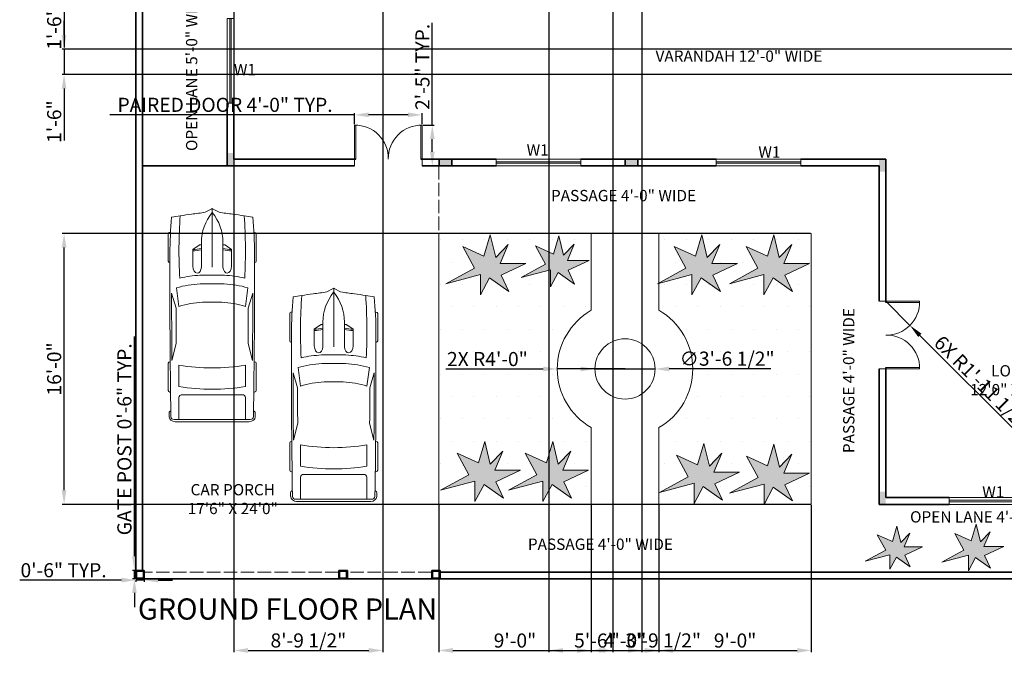
# Model space of a CAD drawing. Units: inches. Extents: x 13878 to 15021, y 3891 to 4810.
# Tile 1 of 3: x 13878 to 14576, y 3891 to 4347. Entities that reach past the tile are written whole.
import ezdxf

# ---------------------------------------------------------------- set-up
doc = ezdxf.new("R2010")
doc.units = ezdxf.units.IN
doc.linetypes.add('ACAD_ISO02W100', pattern=[15, 12, -3])
for name, color, linetype, lineweight in [('A-ANNO-DIMS', 2, 'Continuous', 18), ('A-ANNO-TEXT', 7, 'Continuous', 18), ('A-ANNO-TITL', 7, 'Continuous', 35), ('A-AREA-IDEN', 7, 'Continuous', 18), ('A-COLS', 7, 'Continuous', 35), ('A-COLS-PATT', 7, 'Continuous', 18), ('A-DOOR', 4, 'Continuous', 18), ('A-FLOR-OVHD', 220, 'ACAD_ISO02W100', 18), ('A-GLAZ', 4, 'Continuous', 18), ('A-WALL', 150, 'Continuous', 35), ('C-SITE-GATE', 220, 'ACAD_ISO02W100', 18), ('C-SITE-VEHI', 92, 'Continuous', 13), ('C-SITE-WALL', 150, 'Continuous', 35), ('L-PLNT', 85, 'Continuous', 18), ('L-PLNT-BEDS', 94, 'Continuous', 18)]:
    doc.layers.add(name, color=color, linetype=linetype, lineweight=lineweight)
doc.layers.add('L-PLNT-PATT', color=85, linetype='Continuous', lineweight=13, true_color=0x58ba48)
doc.styles.get("Standard").update_dxf_attribs({"font": 'arial.ttf'})
doc.dimstyles.new('ISO-25', dxfattribs={"dimtxt": 10, "dimasz": 10, "dimexe": 1.25, "dimexo": 0.625, "dimtad": 1, "dimdec": 0, "dimlunit": 3, "dimtxsty": 'Standard', "dimcen": 2.5, "dimadec": 0, "dimazin": 0, "dimtfac": 1, "dimtdec": 0, "dimtmove": 0, "dimatfit": 3, "dimfxl": 1, "dimarcsym": 0})

# ---------------------------------------------------------------- blocks, each defined once
blk = doc.blocks.new('*U2')
for p, q in [((536, 950), (536, 936)), ((1182, 988), (568, 988)), ((1214, 950), (1214, 950)), ((2235, 810), (1899, 912)), ((3412, 904), (3030, 807)), ((3440, 942), (3440, 950)), ((3472, 988), (4087, 988)), ((4119, 950), (4119, 934)), ((1779, 801), (2195, 746)), ((3516, 746), (3994, 746)), ((4179, 670), (4179, -670)), ((4736, 746), (4242, 746)), ((4736, -851), (4736, 851)), ((4785, -832), (4785, 832)), ((756, 241), (1313, 241)), ((816, 241), (816, 283)), ((820, 295), (918, 436)), ((918, 436), (1294, 436)), ((1496, -274), (1496, 274)), ((1690, -267), (1690, 267)), ((4736, -267), (4736, 267)), ((83, 156), (3, 10)), ((2102, 216), (2102, -216)), ((0, 0), (1313, 0)), ((3, -10), (83, -156)), ((756, -241), (1313, -241)), ((816, -241), (816, -283)), ((820, -295), (918, -436)), ((918, -436), (1294, -436)), ((2195, -746), (1779, -801)), ((2235, -810), (1899, -912)), ((3412, -904), (3030, -807)), ((3994, -746), (3516, -746)), ((4242, -746), (4736, -746)), ((536, -950), (536, -936)), ((1182, -988), (568, -988)), ((1214, -950), (1214, -950)), ((3440, -942), (3440, -950)), ((3472, -988), (4087, -988)), ((4119, -950), (4119, -934))]:
    blk.add_line(p, q)
for centre, major_axis, ratio, start_param, end_param in [((6757, -699), (0, 7958), 0.842304, 1.367076, 1.39176), ((1046, -12468), (0, 13417), 0.842304, 0.00281, 0.075598), ((568, 950), (0, -37.6), 0.842304, 3.141593, 4.712389), ((1638, -268113), (0, 269063), 0.842304, -0.013397, 0.002797), ((1182, 950), (0, 37.6), 0.842304, -1.570796, 0), ((1638, -268113), (0, -269025), 0.842304, 3.133765, 3.140441), ((3472, 950), (0, -37.6), 0.842304, 3.141593, 4.712389), ((4087, 950), (0, 37.6), 0.842304, -1.570796, 0), ((4588, 910), (0, 56.4), 0.842304, -0.013017, 1.249894), ((1638, -268131), (0, 269121), 0.842304, -0.013397, -0.013017), ((4673, 851), (0, -75.2), 0.842304, 1.570796, 3.128196), ((4673, 832), (0, -133), 0.842304, 1.570796, 3.128196), ((6583, -699), (0, -7755), 0.842304, 4.528606, 4.561838), ((952, -15087), (0, -15833), 0.842304, 3.096046, 3.200911), ((3414, 137), (0, -2280), 0.842304, 4.449482, 4.652344), ((3436, 137), (0, 2077), 0.842304, 1.245306, 1.50788), ((3800, 71), (0, -2021), 0.842304, 4.372215, 4.640744), ((2433, -93125), (0, -93935), 0.842304, 3.134049, 3.144098), ((434, 0), (0, 3734), 0.842304, 4.511394, 4.913384), ((912, 0), (0, 3734), 0.842304, 4.511394, 4.913384), ((4242, 670), (0, 75.2), 0.842304, 0, 1.570796), ((-5194, 1331), (0, -6374), 0.842304, 1.385369, 1.434372), ((756, -1185), (0, 1427), 0.842304, 0, 0.590319), ((832, 283), (0, 18.8), 0.842304, 0.879714, 1.570796), ((331, 432), (0, 696), 0.842304, 4.435146, 4.718221), ((361, 432), (0, 696), 0.842304, 4.435146, 4.718221), ((1290, 339), (161, -9), 0.603834, -1.395552, 1.581315), ((16, 0), (0, -18.8), 0.842304, 4.131459, 5.293319), ((-5194, -1331), (0, 6374), 0.842304, -1.434372, -1.385369), ((756, 1185), (0, 1427), 0.842304, 2.551274, 3.141593), ((3800, -71), (0, -2021), 0.842304, -1.499151, -1.230623), ((832, -283), (0, -18.8), 0.842304, 4.712389, 5.403472), ((331, -432), (0, -696), 0.842304, 1.564964, 1.848039), ((361, -432), (0, -696), 0.842304, 1.564964, 1.848039), ((3414, -137), (0, -2280), 0.842304, -1.510751, -1.307889), ((3436, -137), (0, -2077), 0.842304, -1.50788, -1.245306), ((6583, 699), (0, 7755), 0.842304, 1.721348, 1.754579), ((6757, 699), (0, 7958), 0.842304, 1.749832, 1.774517), ((952, 15087), (0, -15833), 0.842304, -0.059319, 0.045547), ((2433, 93125), (0, -93935), 0.842304, -0.002505, 0.007544), ((4242, -670), (0, -75.2), 0.842304, 4.712389, 6.283185), ((4673, -851), (0, 75.2), 0.842304, 3.15499, 4.712389), ((4673, -832), (0, -133), 0.842304, 0.013397, 1.570796), ((1046, 12468), (0, -13417), 0.842304, -0.075598, -0.00281), ((568, -950), (0, 37.6), 0.842304, 1.570796, 3.141593), ((1638, 268113), (0, 269063), 0.842304, 3.138796, 3.15499), ((1182, -950), (0, -37.6), 0.842304, 0, 1.570796), ((1638, 268113), (0, -269025), 0.842304, 0.001152, 0.007828), ((3472, -950), (0, -37.6), 0.842304, -1.570796, 0), ((4087, -950), (0, 37.6), 0.842304, 3.141593, 4.712389), ((4588, -910), (0, -56.4), 0.842304, -1.249894, 0.013017), ((1638, 268131), (0, 269121), 0.842304, 3.15461, 3.15499)]:
    blk.add_ellipse(centre, major_axis=major_axis, ratio=ratio, start_param=start_param, end_param=end_param)
at = {"extrusion": (0, 0, -1)}
blk.add_ellipse((1290, -339), major_axis=(161, 9), ratio=0.603834, start_param=-1.395552, end_param=1.581315, dxfattribs=at)
blk = doc.blocks.new('DOOR-PAIR-48IN')
for p, q in [((0, 48), (4.8, 48)), ((4.8, 48), (28.8, 48)), ((4.8, 47), (28.8, 47)), ((4.8, 1), (28.8, 1)), ((0, 0), (4.8, 0)), ((4.8, 0), (28.8, 0))]:
    blk.add_line(p, q)
for centre, start, end in [((5.3, 47.5), 268.78112, 1.21888), ((5.3, 0.5), 358.78112, 91.21888)]:
    blk.add_arc(centre, 23.51, start, end)
blk = doc.blocks.new('WINDOW-W1-60IN')
for p, q in [((0, 0), (0, 4.8)), ((0, 4.8), (60, 4.8)), ((0, 2.9), (60, 2.9)), ((0, 1.9), (60, 1.9)), ((60, 0), (60, 4.8)), ((0, 0), (60, 0))]:
    blk.add_line(p, q)
blk = doc.blocks.new('POST-GATE-6IN')
for p, q in [((6, 6), (0, 6)), ((0, 6), (0, 0)), ((5.5, 5.5), (0.5, 5.5)), ((0.5, 5.5), (0.5, 0.5)), ((0.5, 0.5), (5.5, 0.5)), ((5.5, 0.5), (5.5, 5.5)), ((6, 0), (6, 6)), ((0, 0), (6, 0))]:
    blk.add_line(p, q)
blk = doc.blocks.new('COLUMN-RECT-OUTLINED')
h = blk.add_hatch(color=256)
h.dxf.hatch_style = 1
h.paths.add_polyline_path([(9, 0), (9, 4.8), (0, 4.8), (0, 0)])
for p, q in [((0, 4.8), (0, 0)), ((9, 4.8), (0, 4.8)), ((9, 0), (9, 4.8)), ((0, 0), (9, 0))]:
    blk.add_line(p, q)
blk = doc.blocks.new('COLUMN-RECT-SOLID')
h = blk.add_hatch(color=256)
h.dxf.hatch_style = 1
h.paths.add_polyline_path([(0, 0), (4.8, 0), (4.8, 9), (0, 9)])
blk = doc.blocks.new('*D22')
at = {"layer": 'A-ANNO-DIMS', "color": 0, "lineweight": -2, "ltscale": 2, "transparency": 16777216}
for p, q in [((13959.74, 3966.66), (13959.74, 4122.53)), ((13960.01, 3956.66), (13958.49, 3956.66)), ((13959.74, 3950.66), (13959.74, 3956.66)), ((13960.01, 3950.66), (13958.49, 3950.66)), ((13959.74, 3940.66), (13959.74, 3930.66))]:
    blk.add_line(p, q, dxfattribs=at)
at = {"layer": 'A-ANNO-DIMS', "color": 0, "ltscale": 2, "transparency": 16777216}
for points in [[(13958.07, 3966.66), (13961.4, 3966.66), (13959.74, 3956.66)], [(13958.07, 3940.66), (13961.4, 3940.66), (13959.74, 3950.66)]]:
    blk.add_solid(points, dxfattribs=at)
at = {"layer": 'Defpoints', "color": 0, "ltscale": 2, "transparency": 16777216}
for p in [(13959.74, 3956.66), (13960.64, 3956.66), (13960.64, 3950.66)]:
    blk.add_point(p, dxfattribs=at)
at = {"layer": 'A-ANNO-DIMS', "color": 0, "ltscale": 2, "transparency": 16777216, "insert": (13953.94, 4049.6), "char_height": 10, "attachment_point": 5, "rotation": 90}
blk.add_mtext('GATE POST 0\'-6" TYP.', dxfattribs=at)
blk = doc.blocks.new('*D23')
at = {"layer": 'A-ANNO-DIMS', "color": 0, "lineweight": -2, "ltscale": 2, "transparency": 16777216}
for p, q in [((13950.64, 3949.76), (13878.43, 3949.76)), ((13960.64, 3950.03), (13960.64, 3948.51)), ((13966.64, 3949.76), (13960.64, 3949.76)), ((13966.64, 3950.03), (13966.64, 3948.51)), ((13976.64, 3949.76), (13986.64, 3949.76))]:
    blk.add_line(p, q, dxfattribs=at)
at = {"layer": 'A-ANNO-DIMS', "color": 0, "ltscale": 2, "transparency": 16777216}
for points in [[(13950.64, 3951.43), (13950.64, 3948.09), (13960.64, 3949.76)], [(13976.64, 3951.43), (13976.64, 3948.09), (13966.64, 3949.76)]]:
    blk.add_solid(points, dxfattribs=at)
at = {"layer": 'Defpoints', "color": 0, "ltscale": 2, "transparency": 16777216}
for p in [(13960.64, 3950.66), (13960.64, 3949.76), (13966.64, 3950.66)]:
    blk.add_point(p, dxfattribs=at)
at = {"layer": 'A-ANNO-DIMS', "color": 0, "ltscale": 2, "transparency": 16777216, "insert": (13909.54, 3955.49), "char_height": 10, "attachment_point": 5}
blk.add_mtext('0\'-6" TYP.', dxfattribs=at)
blk = doc.blocks.new('*D34')
at = {"layer": 'A-ANNO-DIMS', "color": 0, "lineweight": -2, "ltscale": 2, "transparency": 16777216}
for p, q in [((14115.67, 4279.6), (13942.28, 4279.6)), ((14115.67, 4273.02), (14115.67, 4280.85)), ((14153.67, 4279.6), (14125.67, 4279.6)), ((14163.67, 4273.02), (14163.67, 4280.85))]:
    blk.add_line(p, q, dxfattribs=at)
at = {"layer": 'A-ANNO-DIMS', "color": 0, "ltscale": 2, "transparency": 16777216}
for points in [[(14125.67, 4281.26), (14125.67, 4277.93), (14115.67, 4279.6)], [(14153.67, 4281.26), (14153.67, 4277.93), (14163.67, 4279.6)]]:
    blk.add_solid(points, dxfattribs=at)
at = {"layer": 'Defpoints', "color": 0, "ltscale": 2, "transparency": 16777216}
for p in [(14115.67, 4279.6), (14115.67, 4272.4), (14163.67, 4272.4)]:
    blk.add_point(p, dxfattribs=at)
at = {"layer": 'A-ANNO-DIMS', "color": 0, "ltscale": 2, "transparency": 16777216, "insert": (14023.98, 4285.4), "char_height": 10, "attachment_point": 5}
blk.add_mtext('PAIRED DOOR 4\'-0" TYP.', dxfattribs=at)
blk = doc.blocks.new('*D35')
at = {"layer": 'A-ANNO-DIMS', "color": 0, "lineweight": -2, "ltscale": 2, "transparency": 16777216}
for p, q in [((14170.87, 4272.4), (14170.87, 4344.77)), ((14164.3, 4272.4), (14172.12, 4272.4)), ((14170.87, 4253.46), (14170.87, 4262.4)), ((14164.3, 4243.46), (14172.12, 4243.46))]:
    blk.add_line(p, q, dxfattribs=at)
at = {"layer": 'A-ANNO-DIMS', "color": 0, "ltscale": 2, "transparency": 16777216}
for points in [[(14169.2, 4262.4), (14172.54, 4262.4), (14170.87, 4272.4)], [(14169.2, 4253.46), (14172.54, 4253.46), (14170.87, 4243.46)]]:
    blk.add_solid(points, dxfattribs=at)
at = {"layer": 'Defpoints', "color": 0, "ltscale": 2, "transparency": 16777216}
for p in [(14163.67, 4272.4), (14170.87, 4272.4), (14163.67, 4243.46)]:
    blk.add_point(p, dxfattribs=at)
at = {"layer": 'A-ANNO-DIMS', "color": 0, "ltscale": 2, "transparency": 16777216, "insert": (14165.14, 4313.58), "char_height": 10, "attachment_point": 5, "rotation": 90}
blk.add_mtext('2\'-5" TYP.', dxfattribs=at)
blk = doc.blocks.new('*D36')
at = {"layer": 'A-ANNO-DIMS', "color": 0, "lineweight": -2, "ltscale": 2, "transparency": 16777216}
for p, q in [((14030.24, 4466.43), (14030.24, 3898.66)), ((14135.84, 4466.43), (14135.84, 3898.66)), ((14040.24, 3899.91), (14125.84, 3899.91))]:
    blk.add_line(p, q, dxfattribs=at)
at = {"layer": 'A-ANNO-DIMS', "color": 0, "ltscale": 2, "transparency": 16777216}
for points in [[(14040.24, 3901.58), (14040.24, 3898.24), (14030.24, 3899.91)], [(14125.84, 3901.58), (14125.84, 3898.24), (14135.84, 3899.91)]]:
    blk.add_solid(points, dxfattribs=at)
at = {"layer": 'Defpoints', "color": 0, "ltscale": 2, "transparency": 16777216}
for p in [(14030.24, 4467.06), (14135.84, 4467.06), (14135.84, 3899.91)]:
    blk.add_point(p, dxfattribs=at)
at = {"layer": 'A-ANNO-DIMS', "color": 0, "ltscale": 2, "transparency": 16777216, "insert": (14083.04, 3905.71), "char_height": 10, "attachment_point": 5}
blk.add_mtext('8\'-9 1/2"', dxfattribs=at)
blk = doc.blocks.new('*D38')
at = {"layer": 'A-ANNO-DIMS', "color": 0, "lineweight": -2, "ltscale": 2, "transparency": 16777216}
for p, q in [((14253.44, 4612.43), (14253.44, 3898.66)), ((14319.44, 4612.43), (14319.44, 3898.66)), ((14263.44, 3899.91), (14309.44, 3899.91))]:
    blk.add_line(p, q, dxfattribs=at)
at = {"layer": 'A-ANNO-DIMS', "color": 0, "ltscale": 2, "transparency": 16777216}
for points in [[(14263.44, 3901.58), (14263.44, 3898.24), (14253.44, 3899.91)], [(14309.44, 3901.58), (14309.44, 3898.24), (14319.44, 3899.91)]]:
    blk.add_solid(points, dxfattribs=at)
at = {"layer": 'Defpoints', "color": 0, "ltscale": 2, "transparency": 16777216}
for p in [(14253.44, 4613.06), (14319.44, 4613.06), (14319.44, 3899.91)]:
    blk.add_point(p, dxfattribs=at)
at = {"layer": 'A-ANNO-DIMS', "color": 0, "ltscale": 2, "transparency": 16777216, "insert": (14286.44, 3905.64), "char_height": 10, "attachment_point": 5}
blk.add_mtext('5\'-6"', dxfattribs=at)
blk = doc.blocks.new('*D39')
at = {"layer": 'A-ANNO-DIMS', "color": 0, "lineweight": -2, "ltscale": 2, "transparency": 16777216}
for p, q in [((14253.44, 4396.43), (14253.44, 3898.66)), ((14298.9, 4396.43), (14298.9, 3898.66)), ((14263.44, 3899.91), (14288.9, 3899.91)), ((14298.9, 3899.91), (14360.03, 3899.91))]:
    blk.add_line(p, q, dxfattribs=at)
at = {"layer": 'A-ANNO-DIMS', "color": 0, "ltscale": 2, "transparency": 16777216}
for points in [[(14263.44, 3901.58), (14263.44, 3898.24), (14253.44, 3899.91)], [(14288.9, 3901.58), (14288.9, 3898.24), (14298.9, 3899.91)]]:
    blk.add_solid(points, dxfattribs=at)
at = {"layer": 'Defpoints', "color": 0, "ltscale": 2, "transparency": 16777216}
for p in [(14253.44, 4397.06), (14298.9, 4397.06), (14298.9, 3899.91)]:
    blk.add_point(p, dxfattribs=at)
at = {"layer": 'A-ANNO-DIMS', "color": 0, "ltscale": 2, "transparency": 16777216, "insert": (14334.46, 3905.71), "char_height": 10, "attachment_point": 5}
blk.add_mtext('3\'-9 1/2"', dxfattribs=at)
blk = doc.blocks.new('*D40')
at = {"layer": 'A-ANNO-DIMS', "color": 0, "lineweight": -2, "ltscale": 2, "transparency": 16777216}
for p, q in [((13909.89, 4402.26), (13909.89, 4412.26)), ((14838.41, 4392.26), (13908.64, 4392.26)), ((13909.89, 4392.26), (13909.89, 4374.26)), ((14838.41, 4374.26), (13908.64, 4374.26)), ((13909.89, 4364.26), (13909.89, 4327.37))]:
    blk.add_line(p, q, dxfattribs=at)
at = {"layer": 'A-ANNO-DIMS', "color": 0, "ltscale": 2, "transparency": 16777216}
for points in [[(13908.22, 4402.26), (13911.55, 4402.26), (13909.89, 4392.26)], [(13908.22, 4364.26), (13911.55, 4364.26), (13909.89, 4374.26)]]:
    blk.add_solid(points, dxfattribs=at)
at = {"layer": 'Defpoints', "color": 0, "ltscale": 2, "transparency": 16777216}
for p in [(14839.04, 4392.26), (13909.89, 4374.26), (14839.04, 4374.26)]:
    blk.add_point(p, dxfattribs=at)
at = {"layer": 'A-ANNO-DIMS', "color": 0, "ltscale": 2, "transparency": 16777216, "insert": (13904.16, 4340.81), "char_height": 10, "attachment_point": 5, "rotation": 90}
blk.add_mtext('1\'-6"', dxfattribs=at)
blk = doc.blocks.new('*D41')
at = {"layer": 'A-ANNO-DIMS', "color": 0, "lineweight": -2, "ltscale": 2, "transparency": 16777216}
for p, q in [((13909.89, 4336.26), (13909.89, 4346.26)), ((14838.41, 4326.26), (13908.64, 4326.26)), ((13909.89, 4326.26), (13909.89, 4308.26)), ((14838.41, 4308.26), (13908.64, 4308.26)), ((13909.89, 4298.26), (13909.89, 4261.37))]:
    blk.add_line(p, q, dxfattribs=at)
at = {"layer": 'A-ANNO-DIMS', "color": 0, "ltscale": 2, "transparency": 16777216}
for points in [[(13908.22, 4336.26), (13911.55, 4336.26), (13909.89, 4326.26)], [(13908.22, 4298.26), (13911.55, 4298.26), (13909.89, 4308.26)]]:
    blk.add_solid(points, dxfattribs=at)
at = {"layer": 'Defpoints', "color": 0, "ltscale": 2, "transparency": 16777216}
for p in [(14839.04, 4326.26), (13909.89, 4308.26), (14839.04, 4308.26)]:
    blk.add_point(p, dxfattribs=at)
at = {"layer": 'A-ANNO-DIMS', "color": 0, "ltscale": 2, "transparency": 16777216, "insert": (13904.16, 4274.81), "char_height": 10, "attachment_point": 5, "rotation": 90}
blk.add_mtext('1\'-6"', dxfattribs=at)
blk = doc.blocks.new('*D42')
at = {"layer": 'A-ANNO-DIMS', "color": 0, "lineweight": -2, "ltscale": 2, "transparency": 16777216}
for p, q in [((14175.44, 4002.83), (14175.44, 3898.66)), ((14283.44, 4002.83), (14283.44, 3898.66)), ((14185.44, 3899.91), (14273.44, 3899.91))]:
    blk.add_line(p, q, dxfattribs=at)
at = {"layer": 'A-ANNO-DIMS', "color": 0, "ltscale": 2, "transparency": 16777216}
for points in [[(14185.44, 3901.58), (14185.44, 3898.24), (14175.44, 3899.91)], [(14273.44, 3901.58), (14273.44, 3898.24), (14283.44, 3899.91)]]:
    blk.add_solid(points, dxfattribs=at)
at = {"layer": 'Defpoints', "color": 0, "ltscale": 2, "transparency": 16777216}
for p in [(14175.44, 4003.46), (14283.44, 4003.46), (14283.44, 3899.91)]:
    blk.add_point(p, dxfattribs=at)
at = {"layer": 'A-ANNO-DIMS', "color": 0, "ltscale": 2, "transparency": 16777216, "insert": (14229.44, 3905.64), "char_height": 10, "attachment_point": 5}
blk.add_mtext('9\'-0"', dxfattribs=at)
blk = doc.blocks.new('*D43')
at = {"layer": 'A-ANNO-DIMS', "color": 0, "lineweight": -2, "ltscale": 2, "transparency": 16777216}
for p, q in [((14283.44, 4002.83), (14283.44, 3898.66)), ((14331.44, 4002.83), (14331.44, 3898.66)), ((14293.44, 3899.91), (14321.44, 3899.91))]:
    blk.add_line(p, q, dxfattribs=at)
at = {"layer": 'A-ANNO-DIMS', "color": 0, "ltscale": 2, "transparency": 16777216}
for points in [[(14293.44, 3901.58), (14293.44, 3898.24), (14283.44, 3899.91)], [(14321.44, 3901.58), (14321.44, 3898.24), (14331.44, 3899.91)]]:
    blk.add_solid(points, dxfattribs=at)
at = {"layer": 'Defpoints', "color": 0, "ltscale": 2, "transparency": 16777216}
for p in [(14283.44, 4003.46), (14331.44, 4003.46), (14331.44, 3899.91)]:
    blk.add_point(p, dxfattribs=at)
at = {"layer": 'A-ANNO-DIMS', "color": 0, "ltscale": 2, "transparency": 16777216, "insert": (14307.44, 3905.64), "char_height": 10, "attachment_point": 5}
blk.add_mtext('4\'-0"', dxfattribs=at)
blk = doc.blocks.new('*D44')
at = {"layer": 'A-ANNO-DIMS', "color": 0, "lineweight": -2, "ltscale": 2, "transparency": 16777216}
for p, q in [((14331.44, 4002.83), (14331.44, 3898.66)), ((14439.44, 4002.83), (14439.44, 3898.66)), ((14341.44, 3899.91), (14429.44, 3899.91))]:
    blk.add_line(p, q, dxfattribs=at)
at = {"layer": 'A-ANNO-DIMS', "color": 0, "ltscale": 2, "transparency": 16777216}
for points in [[(14341.44, 3901.58), (14341.44, 3898.24), (14331.44, 3899.91)], [(14429.44, 3901.58), (14429.44, 3898.24), (14439.44, 3899.91)]]:
    blk.add_solid(points, dxfattribs=at)
at = {"layer": 'Defpoints', "color": 0, "ltscale": 2, "transparency": 16777216}
for p in [(14331.44, 4003.46), (14439.44, 4003.46), (14439.44, 3899.91)]:
    blk.add_point(p, dxfattribs=at)
at = {"layer": 'A-ANNO-DIMS', "color": 0, "ltscale": 2, "transparency": 16777216, "insert": (14385.44, 3905.64), "char_height": 10, "attachment_point": 5}
blk.add_mtext('9\'-0"', dxfattribs=at)
blk = doc.blocks.new('*D45')
at = {"layer": 'A-ANNO-DIMS', "color": 0, "lineweight": -2, "ltscale": 2, "transparency": 16777216}
for p, q in [((14438.81, 4195.46), (13908.64, 4195.46)), ((13909.89, 4013.46), (13909.89, 4185.46)), ((14438.81, 4003.46), (13908.64, 4003.46))]:
    blk.add_line(p, q, dxfattribs=at)
at = {"layer": 'A-ANNO-DIMS', "color": 0, "ltscale": 2, "transparency": 16777216}
for points in [[(13908.22, 4185.46), (13911.55, 4185.46), (13909.89, 4195.46)], [(13908.22, 4013.46), (13911.55, 4013.46), (13909.89, 4003.46)]]:
    blk.add_solid(points, dxfattribs=at)
at = {"layer": 'Defpoints', "color": 0, "ltscale": 2, "transparency": 16777216}
for p in [(13909.89, 4195.46), (14439.44, 4195.46), (14439.44, 4003.46)]:
    blk.add_point(p, dxfattribs=at)
at = {"layer": 'A-ANNO-DIMS', "color": 0, "ltscale": 2, "transparency": 16777216, "insert": (13904.16, 4099.46), "char_height": 10, "attachment_point": 5, "rotation": 90}
blk.add_mtext('16\'-0"', dxfattribs=at)
blk = doc.blocks.new('*D46')
at = {"layer": 'A-ANNO-DIMS', "color": 0, "lineweight": -2, "ltscale": 2, "transparency": 16777216}
for p, q in [((14180.38, 4099.46), (14249.44, 4099.46)), ((14307.44, 4099.46), (14259.44, 4099.46))]:
    blk.add_line(p, q, dxfattribs=at)
at = {"layer": 'A-ANNO-DIMS', "color": 0, "ltscale": 2, "transparency": 16777216}
blk.add_solid([(14249.44, 4101.13), (14249.44, 4097.79), (14259.44, 4099.46)], dxfattribs=at)
at = {"layer": 'Defpoints', "color": 0, "ltscale": 2, "transparency": 16777216}
for p in [(14259.44, 4099.46), (14307.44, 4099.46)]:
    blk.add_point(p, dxfattribs=at)
at = {"layer": 'A-ANNO-DIMS', "color": 0, "ltscale": 2, "transparency": 16777216, "insert": (14209.91, 4105.19), "char_height": 10, "attachment_point": 5, "rotation": 359.99979}
blk.add_mtext('2X R4\'-0"', dxfattribs=at)
blk = doc.blocks.new('*D47')
at = {"layer": 'A-ANNO-DIMS', "color": 0, "lineweight": -2, "ltscale": 2, "transparency": 16777216}
for p, q in [((14276.09, 4099.46), (14266.09, 4099.46)), ((14286.09, 4099.46), (14328.79, 4099.46)), ((14410.8, 4099.46), (14338.79, 4099.46))]:
    blk.add_line(p, q, dxfattribs=at)
at = {"layer": 'A-ANNO-DIMS', "color": 0, "ltscale": 2, "transparency": 16777216}
for points in [[(14276.09, 4101.13), (14276.09, 4097.79), (14286.09, 4099.46)], [(14338.79, 4101.13), (14338.79, 4097.79), (14328.79, 4099.46)]]:
    blk.add_solid(points, dxfattribs=at)
at = {"layer": 'Defpoints', "color": 0, "ltscale": 2, "transparency": 16777216}
for p in [(14286.09, 4099.46), (14328.79, 4099.46)]:
    blk.add_point(p, dxfattribs=at)
at = {"layer": 'A-ANNO-DIMS', "color": 0, "ltscale": 2, "transparency": 16777216, "insert": (14379.79, 4105.47), "char_height": 10, "attachment_point": 5, "rotation": 0.00046}
blk.add_mtext('∅3\'-6 1/2"', dxfattribs=at)
blk = doc.blocks.new('*D50')
at = {"layer": 'A-ANNO-DIMS', "color": 0, "lineweight": -2, "ltscale": 2, "transparency": 16777216}
for p, q in [((14492.74, 4146.96), (14509.36, 4130.34)), ((14587.15, 4052.55), (14516.43, 4123.27))]:
    blk.add_line(p, q, dxfattribs=at)
at = {"layer": 'A-ANNO-DIMS', "color": 0, "ltscale": 2, "transparency": 16777216}
blk.add_solid([(14517.61, 4124.45), (14515.25, 4122.09), (14509.36, 4130.34)], dxfattribs=at)
at = {"layer": 'Defpoints', "color": 0, "ltscale": 2, "transparency": 16777216}
for p in [(14492.74, 4146.96), (14509.36, 4130.34)]:
    blk.add_point(p, dxfattribs=at)
at = {"layer": 'A-ANNO-DIMS', "color": 0, "ltscale": 2, "transparency": 16777216, "insert": (14559.42, 4088.47), "char_height": 10, "attachment_point": 5, "rotation": 315.00023}
blk.add_mtext('6X R1\'-11 1/2"', dxfattribs=at)

msp = doc.modelspace()

# ---------------------------------------------------------------- hatches: boundary and pattern name
at = {"layer": 'L-PLNT-PATT'}
h = msp.add_hatch(dxfattribs=at)
h.set_pattern_fill('DOTS', color=256, scale=10)
h.paths.add_polyline_path([(14283.44, 4141.03), (14283.44, 4195.46), (14175.44, 4195.46), (14175.44, 4003.46), (14283.44, 4003.46), (14283.44, 4057.89, -0.57735)])
h.paths.add_polyline_path([(14225.1, 4154.41), (14211.42, 4164.09), (14204.93, 4151.94), (14204.93, 4166.36), (14180.44, 4159.88), (14200.72, 4170.9), (14192.4, 4186.2), (14207.36, 4179.33), (14211.91, 4194.56), (14215.8, 4178.36), (14224.72, 4187.59), (14219.04, 4174.14), (14237.21, 4174.14), (14219.69, 4165.88)], flags=16)
h.paths.add_polyline_path([(14233.76, 4164.32), (14251, 4173.69), (14243.93, 4186.7), (14256.65, 4180.86), (14260.52, 4193.82), (14263.83, 4180.03), (14271.41, 4187.89), (14266.58, 4176.45), (14282.03, 4176.45), (14267.14, 4169.42), (14271.74, 4159.67), (14260.1, 4167.9), (14254.58, 4157.57), (14254.58, 4169.83)], flags=16)
h.paths.add_polyline_path([(14208.03, 4048.13), (14211.93, 4031.92), (14220.85, 4041.16), (14215.17, 4027.71), (14233.33, 4027.71), (14215.82, 4019.44), (14221.23, 4007.98), (14207.55, 4017.66), (14201.06, 4005.5), (14201.06, 4019.93), (14176.57, 4013.45), (14196.84, 4024.47), (14188.53, 4039.77), (14203.49, 4032.89)], flags=16)
h.paths.add_polyline_path([(14256.22, 4048.13), (14260.11, 4031.92), (14269.03, 4041.16), (14263.36, 4027.71), (14281.52, 4027.71), (14264.01, 4019.44), (14269.42, 4007.98), (14255.74, 4017.66), (14249.25, 4005.5), (14249.25, 4019.93), (14224.76, 4013.45), (14245.03, 4024.47), (14236.72, 4039.77), (14251.68, 4032.89)], flags=16)
h = msp.add_hatch(color=256, dxfattribs=at)
h.dxf.hatch_style = 1
h.paths.add_polyline_path([(14211.42, 4164.09), (14225.1, 4154.41), (14219.69, 4165.88), (14237.21, 4174.14), (14219.04, 4174.14), (14224.72, 4187.59), (14215.8, 4178.36), (14211.91, 4194.56), (14207.36, 4179.33), (14192.4, 4186.2), (14200.72, 4170.9), (14180.44, 4159.88), (14204.93, 4166.36), (14204.93, 4151.94)])
h.paths.add_polyline_path([(14260.1, 4167.9), (14271.74, 4159.67), (14267.14, 4169.42), (14282.03, 4176.45), (14266.58, 4176.45), (14271.41, 4187.89), (14263.83, 4180.03), (14260.52, 4193.82), (14256.65, 4180.86), (14243.93, 4186.7), (14251, 4173.69), (14233.76, 4164.32), (14254.58, 4169.83), (14254.58, 4157.57)])
h.paths.add_polyline_path([(14365.73, 4178.36), (14361.84, 4194.56), (14357.3, 4179.33), (14342.33, 4186.2), (14350.65, 4170.9), (14331.44, 4160.46), (14331.44, 4160.16), (14354.86, 4166.36), (14354.86, 4151.94), (14361.35, 4164.09), (14375.03, 4154.41), (14369.62, 4165.88), (14387.14, 4174.14), (14368.97, 4174.14), (14374.65, 4187.59)])
h.paths.add_polyline_path([(14420, 4174.14), (14425.67, 4187.59), (14416.75, 4178.36), (14412.86, 4194.56), (14408.32, 4179.33), (14393.35, 4186.2), (14401.67, 4170.9), (14381.4, 4159.88), (14405.89, 4166.36), (14405.89, 4151.94), (14412.37, 4164.09), (14426.05, 4154.41), (14420.65, 4165.88), (14438.16, 4174.14)])
h.paths.add_polyline_path([(14249.25, 4019.93), (14249.25, 4005.5), (14255.74, 4017.66), (14269.42, 4007.98), (14264.01, 4019.44), (14281.52, 4027.71), (14263.36, 4027.71), (14269.03, 4041.16), (14260.11, 4031.92), (14256.22, 4048.13), (14251.68, 4032.89), (14236.72, 4039.77), (14245.03, 4024.47), (14224.76, 4013.45)])
h.paths.add_polyline_path([(14203.49, 4032.89), (14188.53, 4039.77), (14196.84, 4024.47), (14176.57, 4013.45), (14201.06, 4019.93), (14201.06, 4005.5), (14207.55, 4017.66), (14221.23, 4007.98), (14215.82, 4019.44), (14233.33, 4027.71), (14215.17, 4027.71), (14220.85, 4041.16), (14211.93, 4031.92), (14208.03, 4048.13)])
h.paths.add_polyline_path([(14362.82, 4016.2), (14376.5, 4006.52), (14371.09, 4017.98), (14388.61, 4026.25), (14370.44, 4026.25), (14376.12, 4039.7), (14367.2, 4030.46), (14363.31, 4046.67), (14358.76, 4031.44), (14343.8, 4038.31), (14352.12, 4023.01), (14331.84, 4011.99), (14356.33, 4018.47), (14356.33, 4004.05)])
h.paths.add_polyline_path([(14408.41, 4030.85), (14393.45, 4037.72), (14401.76, 4022.42), (14381.49, 4011.4), (14405.98, 4017.88), (14405.98, 4003.46), (14412.47, 4015.62), (14426.15, 4005.94), (14420.74, 4017.4), (14438.25, 4025.66), (14420.09, 4025.66), (14425.77, 4039.12), (14416.85, 4029.88), (14412.95, 4046.08)])
h.paths.add_polyline_path([(14502.95, 3976.33), (14500.16, 3987.92), (14496.92, 3977.03), (14486.21, 3981.94), (14492.16, 3971), (14477.66, 3963.12), (14495.18, 3967.76), (14495.18, 3957.44), (14499.81, 3966.13), (14509.6, 3959.21), (14505.73, 3967.41), (14518.25, 3973.32), (14505.27, 3973.32), (14509.32, 3982.94)])
h.paths.add_polyline_path([(14552.74, 3977.57), (14541.18, 3982.88), (14547.61, 3971.06), (14531.95, 3962.55), (14550.86, 3967.56), (14550.86, 3956.41), (14555.87, 3965.8), (14566.44, 3958.33), (14562.26, 3967.18), (14575.79, 3973.56), (14561.76, 3973.56), (14566.15, 3983.95), (14559.26, 3976.82), (14556.25, 3989.34)])
h.paths.add_polyline_path([(14605.39, 3973.1), (14587.22, 3963.23), (14609.17, 3969.04), (14609.17, 3956.11), (14614.98, 3967), (14627.25, 3958.33), (14622.4, 3968.6), (14638.1, 3976.01), (14621.82, 3976.01), (14626.9, 3988.07), (14618.91, 3979.79), (14615.42, 3994.31), (14611.35, 3980.66), (14597.94, 3986.82)])
h = msp.add_hatch(dxfattribs=at)
h.set_pattern_fill('DOTS', color=256, scale=10)
h.paths.add_polyline_path([(14439.44, 4195.46), (14331.44, 4195.46), (14331.44, 4160.46), (14350.65, 4170.9), (14342.33, 4186.2), (14357.3, 4179.33), (14361.84, 4194.56), (14365.73, 4178.36), (14374.65, 4187.59), (14368.97, 4174.14), (14387.14, 4174.14), (14369.62, 4165.88), (14375.03, 4154.41), (14361.35, 4164.09), (14354.86, 4151.94), (14354.86, 4166.36), (14331.44, 4160.16), (14331.44, 4141.03, -0.57735), (14331.44, 4057.89), (14331.44, 4003.46), (14405.98, 4003.46), (14405.98, 4017.88), (14381.49, 4011.4), (14401.76, 4022.42), (14393.45, 4037.72), (14408.41, 4030.85), (14412.95, 4046.08), (14416.85, 4029.88), (14425.77, 4039.12), (14420.09, 4025.66), (14438.25, 4025.66), (14420.74, 4017.4), (14426.15, 4005.94), (14412.47, 4015.62), (14405.98, 4003.46), (14439.44, 4003.46)])
h.paths.add_polyline_path([(14381.4, 4159.88), (14401.67, 4170.9), (14393.35, 4186.2), (14408.32, 4179.33), (14412.86, 4194.56), (14416.75, 4178.36), (14425.67, 4187.59), (14420, 4174.14), (14438.16, 4174.14), (14420.65, 4165.88), (14426.05, 4154.41), (14412.37, 4164.09), (14405.89, 4151.94), (14405.89, 4166.36)], flags=16)
h.paths.add_polyline_path([(14363.31, 4046.67), (14367.2, 4030.46), (14376.12, 4039.7), (14370.44, 4026.25), (14388.61, 4026.25), (14371.09, 4017.98), (14376.5, 4006.52), (14362.82, 4016.2), (14356.33, 4004.05), (14356.33, 4018.47), (14331.84, 4011.99), (14352.12, 4023.01), (14343.8, 4038.31), (14358.76, 4031.44)], flags=16)

# ---------------------------------------------------------------- linework, layer by layer
at = {"layer": 'A-DOOR'}
for p, q in [((14487.44, 4147.46), (14492.24, 4147.46)), ((14492.24, 4147.46), (14516.24, 4147.46)), ((14492.24, 4146.46), (14516.24, 4146.46)), ((14492.24, 4123.45), (14492.24, 4123.46)), ((14487.44, 4099.46), (14492.24, 4099.46)), ((14492.24, 4100.46), (14516.24, 4100.46)), ((14492.24, 4099.46), (14516.24, 4099.46))]:
    msp.add_line(p, q, dxfattribs=at)
for centre, radius, start, end in [((14492.74, 4146.96), 23.51, 268.78112, 1.21888), ((14492.74, 4099.96), 23.5, 358.78085, 91.23184)]:
    msp.add_arc(centre, radius, start, end, dxfattribs=at)
at = {"layer": 'A-FLOR-OVHD', "ltscale": 0.8}
msp.add_line((14175.44, 4243.46), (14175.44, 3956.66), dxfattribs=at)
at = {"layer": 'A-GLAZ'}
msp.add_line((14216.1, 4246.36), (14276.1, 4246.36), dxfattribs=at)
at = {"layer": 'A-WALL'}
for p, q in [((14025.44, 4243.46), (14025.44, 4287.86)), ((14030.24, 4248.26), (14030.24, 4287.86)), ((14115.67, 4243.46), (13965.44, 4243.46)), ((14116.67, 4248.26), (14030.24, 4248.26)), ((14216.1, 4248.26), (14162.67, 4248.26)), ((14184.77, 4243.46), (14163.67, 4243.46)), ((14216.1, 4243.46), (14184.77, 4243.46)), ((14371.94, 4248.26), (14276.1, 4248.26)), ((14307.44, 4243.46), (14276.1, 4243.46)), ((14316.44, 4243.46), (14307.44, 4243.46)), ((14371.94, 4243.46), (14316.44, 4243.46)), ((14492.24, 4248.26), (14431.94, 4248.26)), ((14487.44, 4243.46), (14431.94, 4243.46)), ((14487.44, 4147.46), (14487.44, 4243.46)), ((14492.24, 4146.46), (14492.24, 4248.26)), ((14487.44, 4003.46), (14487.44, 4099.46)), ((14492.24, 4008.26), (14492.24, 4100.46)), ((14537.24, 4008.26), (14492.24, 4008.26)), ((14537.24, 4003.46), (14487.44, 4003.46))]:
    msp.add_line(p, q, dxfattribs=at)
at = {"layer": 'C-SITE-GATE', "ltscale": 0.8}
for p, q in [((14104.64, 3955.46), (13966.64, 3955.46)), ((14170.41, 3955.46), (14110.64, 3955.46))]:
    msp.add_line(p, q, dxfattribs=at)
at = {"layer": 'C-SITE-WALL'}
for p, q in [((13960.64, 3950.66), (13960.64, 4670.66)), ((13965.44, 3956.66), (13965.44, 4392.26)), ((13966.64, 3950.66), (13960.64, 3950.66)), ((14176.41, 3950.66), (13966.64, 3950.66)), ((14487.44, 3955.46), (14176.41, 3955.46)), ((14920.64, 3950.66), (14176.41, 3950.66)), ((14642.24, 3955.46), (14487.44, 3955.46))]:
    msp.add_line(p, q, dxfattribs=at)
at = {"layer": 'L-PLNT'}
for p, q in [((14207.36, 4179.33), (14211.91, 4194.56)), ((14211.91, 4194.56), (14215.8, 4178.36)), ((14256.65, 4180.86), (14260.52, 4193.82)), ((14260.52, 4193.82), (14263.83, 4180.03)), ((14357.3, 4179.33), (14361.84, 4194.56)), ((14361.84, 4194.56), (14365.73, 4178.36)), ((14408.32, 4179.33), (14412.86, 4194.56)), ((14412.86, 4194.56), (14416.75, 4178.36)), ((14215.8, 4178.36), (14224.72, 4187.59)), ((14224.72, 4187.59), (14219.04, 4174.14)), ((14263.83, 4180.03), (14271.41, 4187.89)), ((14271.41, 4187.89), (14266.58, 4176.45)), ((14365.73, 4178.36), (14374.65, 4187.59)), ((14374.65, 4187.59), (14368.97, 4174.14)), ((14416.75, 4178.36), (14425.67, 4187.59)), ((14425.67, 4187.59), (14420, 4174.14)), ((14200.72, 4170.9), (14192.4, 4186.2)), ((14192.4, 4186.2), (14207.36, 4179.33)), ((14251, 4173.69), (14243.93, 4186.7)), ((14243.93, 4186.7), (14256.65, 4180.86)), ((14350.65, 4170.9), (14342.33, 4186.2)), ((14342.33, 4186.2), (14357.3, 4179.33)), ((14401.67, 4170.9), (14393.35, 4186.2)), ((14393.35, 4186.2), (14408.32, 4179.33)), ((14219.04, 4174.14), (14237.21, 4174.14)), ((14237.21, 4174.14), (14219.69, 4165.88)), ((14233.76, 4164.32), (14251, 4173.69)), ((14266.58, 4176.45), (14282.03, 4176.45)), ((14282.03, 4176.45), (14267.14, 4169.42)), ((14368.97, 4174.14), (14387.14, 4174.14)), ((14387.14, 4174.14), (14369.62, 4165.88)), ((14420, 4174.14), (14438.16, 4174.14)), ((14438.16, 4174.14), (14420.65, 4165.88)), ((14180.44, 4159.88), (14200.72, 4170.9)), ((14204.93, 4166.36), (14180.44, 4159.88)), ((14204.93, 4151.94), (14204.93, 4166.36)), ((14254.58, 4169.83), (14233.76, 4164.32)), ((14254.58, 4157.57), (14254.58, 4169.83)), ((14260.1, 4167.9), (14254.58, 4157.57)), ((14271.74, 4159.67), (14260.1, 4167.9)), ((14267.14, 4169.42), (14271.74, 4159.67)), ((14330.38, 4159.88), (14350.65, 4170.9)), ((14354.86, 4166.36), (14330.38, 4159.88)), ((14354.86, 4151.94), (14354.86, 4166.36)), ((14381.4, 4159.88), (14401.67, 4170.9)), ((14405.89, 4166.36), (14381.4, 4159.88)), ((14405.89, 4151.94), (14405.89, 4166.36)), ((14211.42, 4164.09), (14204.93, 4151.94)), ((14225.1, 4154.41), (14211.42, 4164.09)), ((14219.69, 4165.88), (14225.1, 4154.41)), ((14361.35, 4164.09), (14354.86, 4151.94)), ((14375.03, 4154.41), (14361.35, 4164.09)), ((14369.62, 4165.88), (14375.03, 4154.41)), ((14412.37, 4164.09), (14405.89, 4151.94)), ((14426.05, 4154.41), (14412.37, 4164.09)), ((14420.65, 4165.88), (14426.05, 4154.41)), ((14203.49, 4032.89), (14208.03, 4048.13)), ((14208.03, 4048.13), (14211.93, 4031.92)), ((14251.68, 4032.89), (14256.22, 4048.13)), ((14256.22, 4048.13), (14260.11, 4031.92)), ((14211.93, 4031.92), (14220.85, 4041.16)), ((14220.85, 4041.16), (14215.17, 4027.71)), ((14260.11, 4031.92), (14269.03, 4041.16)), ((14269.03, 4041.16), (14263.36, 4027.71)), ((14358.76, 4031.44), (14363.31, 4046.67)), ((14363.31, 4046.67), (14367.2, 4030.46)), ((14408.41, 4030.85), (14412.95, 4046.08)), ((14412.95, 4046.08), (14416.85, 4029.88)), ((14196.84, 4024.47), (14188.53, 4039.77)), ((14188.53, 4039.77), (14203.49, 4032.89)), ((14245.03, 4024.47), (14236.72, 4039.77)), ((14236.72, 4039.77), (14251.68, 4032.89)), ((14352.12, 4023.01), (14343.8, 4038.31)), ((14343.8, 4038.31), (14358.76, 4031.44)), ((14367.2, 4030.46), (14376.12, 4039.7)), ((14376.12, 4039.7), (14370.44, 4026.25)), ((14401.76, 4022.42), (14393.45, 4037.72)), ((14393.45, 4037.72), (14408.41, 4030.85)), ((14416.85, 4029.88), (14425.77, 4039.12)), ((14425.77, 4039.12), (14420.09, 4025.66)), ((14215.17, 4027.71), (14233.33, 4027.71)), ((14233.33, 4027.71), (14215.82, 4019.44)), ((14263.36, 4027.71), (14281.52, 4027.71)), ((14281.52, 4027.71), (14264.01, 4019.44)), ((14176.57, 4013.45), (14196.84, 4024.47)), ((14201.06, 4019.93), (14176.57, 4013.45)), ((14201.06, 4005.5), (14201.06, 4019.93)), ((14215.82, 4019.44), (14221.23, 4007.98)), ((14224.76, 4013.45), (14245.03, 4024.47)), ((14249.25, 4019.93), (14224.76, 4013.45)), ((14249.25, 4005.5), (14249.25, 4019.93)), ((14264.01, 4019.44), (14269.42, 4007.98)), ((14331.84, 4011.99), (14352.12, 4023.01)), ((14370.44, 4026.25), (14388.61, 4026.25)), ((14388.61, 4026.25), (14371.09, 4017.98)), ((14381.49, 4011.4), (14401.76, 4022.42)), ((14420.09, 4025.66), (14438.25, 4025.66)), ((14438.25, 4025.66), (14420.74, 4017.4)), ((14207.55, 4017.66), (14201.06, 4005.5)), ((14221.23, 4007.98), (14207.55, 4017.66)), ((14255.74, 4017.66), (14249.25, 4005.5)), ((14269.42, 4007.98), (14255.74, 4017.66)), ((14356.33, 4018.47), (14331.84, 4011.99)), ((14356.33, 4004.05), (14356.33, 4018.47)), ((14362.82, 4016.2), (14356.33, 4004.05)), ((14376.5, 4006.52), (14362.82, 4016.2)), ((14371.09, 4017.98), (14376.5, 4006.52)), ((14405.98, 4017.88), (14381.49, 4011.4)), ((14405.98, 4003.46), (14405.98, 4017.88)), ((14412.47, 4015.62), (14405.98, 4003.46)), ((14426.15, 4005.94), (14412.47, 4015.62)), ((14420.74, 4017.4), (14426.15, 4005.94)), ((14496.92, 3977.03), (14500.16, 3987.92)), ((14500.16, 3987.92), (14502.95, 3976.33)), ((14552.74, 3977.57), (14556.25, 3989.34)), ((14556.25, 3989.34), (14559.26, 3976.82)), ((14492.16, 3971), (14486.21, 3981.94)), ((14486.21, 3981.94), (14496.92, 3977.03)), ((14502.95, 3976.33), (14509.32, 3982.94)), ((14509.32, 3982.94), (14505.27, 3973.32)), ((14547.61, 3971.06), (14541.18, 3982.88)), ((14541.18, 3982.88), (14552.74, 3977.57)), ((14559.26, 3976.82), (14566.15, 3983.95)), ((14566.15, 3983.95), (14561.76, 3973.56)), ((14477.66, 3963.12), (14492.16, 3971)), ((14505.27, 3973.32), (14518.25, 3973.32)), ((14518.25, 3973.32), (14505.73, 3967.41)), ((14531.95, 3962.55), (14547.61, 3971.06)), ((14561.76, 3973.56), (14575.79, 3973.56)), ((14575.79, 3973.56), (14562.26, 3967.18)), ((14495.18, 3967.76), (14477.66, 3963.12)), ((14495.18, 3957.44), (14495.18, 3967.76)), ((14499.81, 3966.13), (14495.18, 3957.44)), ((14509.6, 3959.21), (14499.81, 3966.13)), ((14505.73, 3967.41), (14509.6, 3959.21)), ((14550.86, 3967.56), (14531.95, 3962.55)), ((14550.86, 3956.41), (14550.86, 3967.56)), ((14555.87, 3965.8), (14550.86, 3956.41)), ((14566.44, 3958.33), (14555.87, 3965.8)), ((14562.26, 3967.18), (14566.44, 3958.33))]:
    msp.add_line(p, q, dxfattribs=at)
at = {"layer": 'L-PLNT-BEDS'}
for p, q in [((14175.44, 4003.46), (14175.44, 4195.46)), ((14283.44, 4195.46), (14175.44, 4195.46)), ((14283.44, 4195.46), (14283.44, 4141.03)), ((14439.44, 4195.46), (14331.44, 4195.46)), ((14331.44, 4195.46), (14331.44, 4141.03)), ((14439.44, 4003.46), (14439.44, 4195.46)), ((14283.44, 4057.89), (14283.44, 4003.46)), ((14331.44, 4057.89), (14331.44, 4003.46)), ((14283.44, 4003.46), (14175.44, 4003.46)), ((14439.44, 4003.46), (14331.44, 4003.46))]:
    msp.add_line(p, q, dxfattribs=at)
msp.add_lwpolyline([(14331.44, 4141.03), (14331.44, 4195.46), (14439.44, 4195.46), (14439.44, 4003.46), (14331.44, 4003.46), (14331.44, 4057.89)], dxfattribs=at)
msp.add_circle((14307.44, 4099.46), 21.35, dxfattribs=at)
for start, end in [(120, 240), (300, 60)]:
    msp.add_arc((14307.44, 4099.46), 48, start, end, dxfattribs=at)

# ---------------------------------------------------------------- block references
at = {"layer": 'A-COLS'}
for name, p in [('COLUMN-RECT-OUTLINED', (14175.77, 4243.46)), ('COLUMN-RECT-OUTLINED', (14307.44, 4243.46)), ('POST-GATE-6IN', (14104.64, 3950.66))]:
    msp.add_blockref(name, p, dxfattribs=at)
at = {"layer": 'A-COLS', "rotation": 89.99999999996525}
for p in [(13966.64, 3950.66), (14176.41, 3950.66)]:
    msp.add_blockref('POST-GATE-6IN', p, dxfattribs=at)
at = {"layer": 'A-COLS-PATT'}
for p in [(14025.44, 4243.47), (14487.44, 4239.31), (14487.44, 4003.48)]:
    msp.add_blockref('COLUMN-RECT-SOLID', p, dxfattribs=at)
at = {"layer": 'A-DOOR', "rotation": 90.00000000000452}
msp.add_blockref('DOOR-PAIR-48IN', (14163.67, 4243.46), dxfattribs=at)
at = {"layer": 'A-GLAZ'}
for p, rotation in [((14030.24, 4287.86), 89.99999999999301), ((14276.1, 4248.26), 180), ((14431.94, 4248.26), 180), ((14597.24, 4008.26), 180)]:
    msp.add_blockref('WINDOW-W1-60IN', p, dxfattribs=dict(at, rotation=rotation))
at = {"layer": 'C-SITE-VEHI', "xscale": 0.0315695346537715, "yscale": 0.0315695346537715, "zscale": 0.0315695346537715, "rotation": 270}
for p in [(14014.86, 4213.14), (14100.96, 4156.64)]:
    msp.add_blockref('*U2', p, dxfattribs=at)

# ---------------------------------------------------------------- texts
at = {"layer": 'A-ANNO-TEXT', "char_height": 8, "attachment_point": 1}
for insert in [(14030.24, 4315.7), (14237.72, 4258.67), (14401.94, 4257.2), (14560.59, 4016.29)]:
    msp.add_mtext_dynamic_manual_height_columns('W1', width=16.3853, gutter_width=12.5, heights=[0], dxfattribs=dict(at, insert=insert))
at = {"layer": 'A-ANNO-TITL', "insert": (13962.2, 3936.79), "char_height": 15, "attachment_point": 1}
msp.add_mtext_dynamic_manual_height_columns('GROUND FLOOR PLAN', width=275.3527, gutter_width=12.5, heights=[0], dxfattribs=at)
at = {"layer": 'A-AREA-IDEN', "char_height": 8, "attachment_point": 1, "rotation": 90}
for s, insert in [('OPEN LANE 5\'-0" WIDE', (13996.3, 4253.96)), ('PASSAGE 4\'-0" WIDE', (14462, 4039.79))]:
    msp.add_mtext_dynamic_manual_height_columns(s, width=379.1288, gutter_width=12.5, heights=[0], dxfattribs=dict(at, insert=insert))
at = {"layer": 'A-AREA-IDEN', "char_height": 8, "attachment_point": 1}
for s, width, insert in [('VARANDAH 12\'-0" WIDE', 379.1288, (14329.05, 4325.21)), ('PASSAGE 4\'-0" WIDE', 379.1288, (14254.95, 4226.37)), ('\\pxqc;LOBBY\\P12\'0" X 13\'6"', 129.4248, (14519.29, 4102.16)), ('\\pxqc;CAR PORCH\\P17\'6" X 24\'0"', 66.7259, (13996.09, 4017.87)), ('OPEN LANE 4\'-0" WIDE', 379.1288, (14509.45, 3998.61)), ('PASSAGE 4\'-0" WIDE', 379.1288, (14238.58, 3979.21))]:
    msp.add_mtext_dynamic_manual_height_columns(s, width=width, gutter_width=12.5, heights=[0], dxfattribs=dict(at, insert=insert))

# ---------------------------------------------------------------- dimensions: what is measured, and where the dimension line sits
at = {"layer": 'A-ANNO-DIMS', "ltscale": 2}
for base, p1, p2, picture, middle in [((14319.44, 3899.91), (14253.44, 4613.06), (14319.44, 4613.06), '*D38', (14286.44, 3905.64)), ((14135.84, 3899.91), (14030.24, 4467.06), (14135.84, 4467.06), '*D36', (14083.04, 3905.71)), ((14298.9, 3899.91), (14253.44, 4397.06), (14298.9, 4397.06), '*D39', (14334.46, 3905.71)), ((14283.44, 3899.91), (14175.44, 4003.46), (14283.44, 4003.46), '*D42', (14229.44, 3905.64)), ((14331.44, 3899.91), (14283.44, 4003.46), (14331.44, 4003.46), '*D43', (14307.44, 3905.64)), ((14439.44, 3899.91), (14331.44, 4003.46), (14439.44, 4003.46), '*D44', (14385.44, 3905.64))]:
    dim = msp.add_linear_dim(base=base, p1=p1, p2=p2, dimstyle='ISO-25', override={"dimdec": 1, "dimlfac": 1, "dimrnd": 0, "dimzin": 1, "dimdsep": 46, "dimlunit": 4, "dimfrac": 2}, dxfattribs=at)
    dim.commit()
    dim.dimension.update_dxf_attribs({"geometry": picture, "text_midpoint": middle})
for base, p1, p2, picture, middle in [((13909.89, 4374.26), (14839.04, 4392.26), (14839.04, 4374.26), '*D40', (13904.16, 4340.81)), ((13909.89, 4308.26), (14839.04, 4326.26), (14839.04, 4308.26), '*D41', (13904.16, 4274.81)), ((13909.89, 4195.46), (14439.44, 4003.46), (14439.44, 4195.46), '*D45', (13904.16, 4099.46))]:
    dim = msp.add_linear_dim(base=base, p1=p1, p2=p2, angle=90, dimstyle='ISO-25', override={"dimdec": 1, "dimlfac": 1, "dimrnd": 0, "dimzin": 1, "dimdsep": 46, "dimlunit": 4, "dimfrac": 2}, dxfattribs=at)
    dim.commit()
    dim.dimension.update_dxf_attribs({"geometry": picture, "text_midpoint": middle})
for base, p1, p2, angle, text, picture, middle in [((14170.87, 4272.4), (14163.67, 4243.46), (14163.67, 4272.4), 90, '<> TYP.', '*D35', (14165.14, 4313.58)), ((14115.67, 4279.6), (14163.67, 4272.4), (14115.67, 4272.4), 180, 'PAIRED DOOR <> TYP.', '*D34', (14023.98, 4285.4)), ((13959.74, 3956.66), (13960.64, 3950.66), (13960.64, 3956.66), 90, 'GATE POST <> TYP.', '*D22', (13953.94, 4049.6)), ((13960.64, 3949.76), (13966.64, 3950.66), (13960.64, 3950.66), 180, '<> TYP.', '*D23', (13909.54, 3955.49))]:
    dim = msp.add_linear_dim(base=base, p1=p1, p2=p2, angle=angle, text=text, dimstyle='ISO-25', override={"dimdec": 1, "dimlfac": 1, "dimrnd": 0, "dimzin": 1, "dimdsep": 46, "dimlunit": 4, "dimfrac": 2}, dxfattribs=at)
    dim.commit()
    dim.dimension.update_dxf_attribs({"geometry": picture, "text_midpoint": middle})
for center, mpoint, text, picture, middle in [((14492.74, 4146.96), (14509.36, 4130.34), '6X <>', '*D50', (14559.42, 4088.47)), ((14307.44, 4099.46), (14259.44, 4099.46), '2X <>', '*D46', (14209.91, 4105.19))]:
    dim = msp.add_radius_dim(center=center, mpoint=mpoint, text=text, dimstyle='ISO-25', override={"dimdec": 1, "dimlfac": 1, "dimrnd": 0, "dimzin": 1, "dimdsep": 46, "dimlunit": 4, "dimfrac": 2}, dxfattribs=at)
    dim.commit()
    dim.dimension.update_dxf_attribs({"geometry": picture, "text_midpoint": middle})
dim = msp.add_diameter_dim_2p(p1=(14286.09, 4099.46), p2=(14328.79, 4099.46), dimstyle='ISO-25', override={"dimdec": 1, "dimlfac": 1, "dimrnd": 0, "dimzin": 1, "dimdsep": 46, "dimlunit": 4, "dimfrac": 2}, dxfattribs=at)
dim.commit()
dim.dimension.update_dxf_attribs({"geometry": '*D47', "text_midpoint": (14379.79, 4099.46), "dimtype": 163})

doc.saveas('drawing.dxf')
